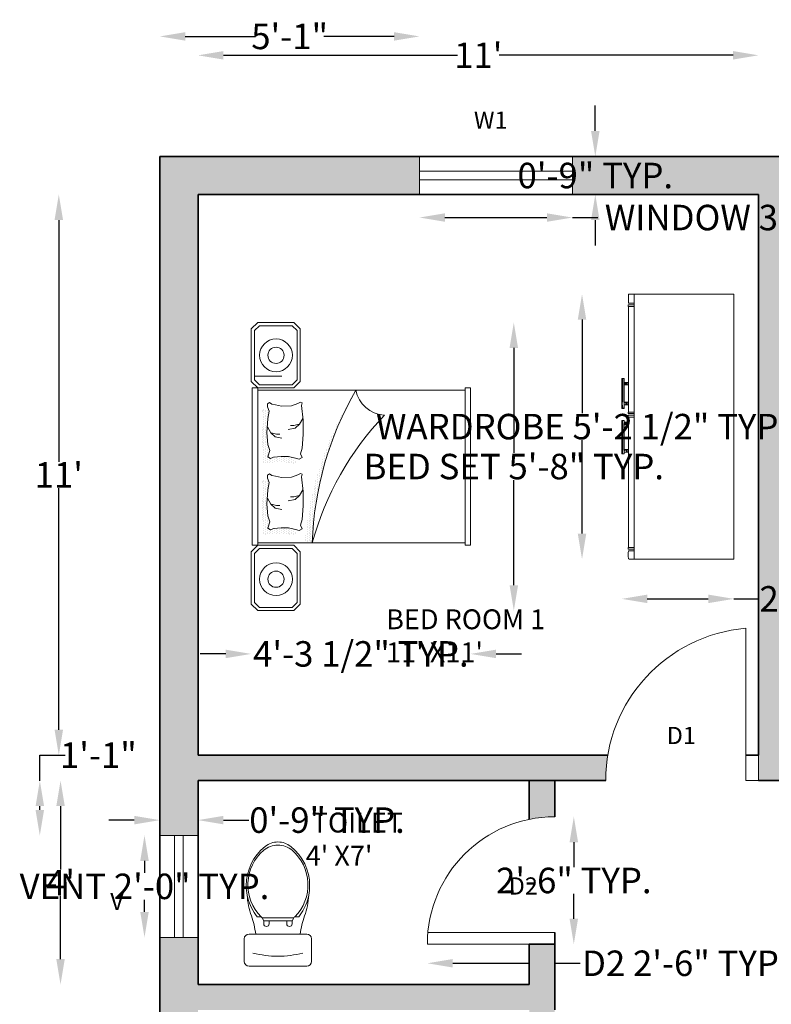
# Model space of a CAD drawing. Units: inches. Extents: x 2178 to 3409, y 1711 to 2279.
# Tile 3 of 8: x 2191 to 2368, y 2047 to 2279. Entities that reach past the tile are written whole.
import ezdxf

# ---------------------------------------------------------------- set-up
doc = ezdxf.new("R2010")
doc.units = ezdxf.units.IN
for name, color, linetype, lineweight in [('A-ANNO-DIMS', 2, 'Continuous', 18), ('A-ANNO-IDEN', 3, 'Continuous', 18), ('A-AREA-IDEN', 7, 'Continuous', 18), ('A-DOOR', 4, 'Continuous', 18), ('A-FURN', 8, 'Continuous', 18), ('A-GLAZ', 4, 'Continuous', 18), ('A-WALL', 7, 'Continuous', 35), ('A-WALL-PATT', 252, 'Continuous', 13), ('WC-Detail_dwgmodels.com', 240, 'Continuous', 13), ('WC-Outline_dwgmodels.com', 250, 'Continuous', 18)]:
    doc.layers.add(name, color=color, linetype=linetype, lineweight=lineweight)
doc.styles.get("Standard").update_dxf_attribs({"font": 'arial.ttf'})
doc.dimstyles.get("Standard").update_dxf_attribs({"dimtxt": 6, "dimasz": 6, "dimexe": 0.18, "dimexo": 0.0625, "dimgap": 0.09, "dimtad": 0, "dimtih": 1, "dimtoh": 1, "dimdec": 4, "dimzin": 0, "dimdsep": 46, "dimlunit": 4, "dimtxsty": 'Standard', "dimcen": 0.09, "dimse1": 1, "dimse2": 1, "dimadec": 0, "dimazin": 0, "dimtfac": 1, "dimtdec": 4, "dimtofl": 0, "dimtmove": 0, "dimatfit": 3, "dimfxl": 1, "dimtolj": 1, "dimtzin": 0, "dimarcsym": 0})
pattern_1 = [(90, (3285.2007, -5256.0159), (-0.408110856, 0.204055428), [0, -0.408110856])]
pattern_2 = [(2e-12, (221.4576, -2145.7372), (1.73228346, -0.78740157), [11.8110236, -1.574803, 3.937008, -0.7874016]), (2e-12, (222.5049, -2146.1309), (-0.7874016, -1.0472441), [2.3622047, -0.2598425, 4.7244094, -0.5905512]), (2e-12, (221.8513, -2146.4065), (4.09448819, -0.52755906), [6.2992126, -1.1023622, 3.1496063, -0.7874016])]

# ---------------------------------------------------------------- blocks, each defined once
blk = doc.blocks.new('*D11')
at = {"layer": 'A-ANNO-DIMS', "color": 0, "lineweight": -2, "transparency": 16777216}
for p, q in [((2200.28, 2232.04), (2200.28, 2175.14)), ((2200.28, 2112.04), (2200.28, 2168.94))]:
    blk.add_line(p, q, dxfattribs=at)
at = {"layer": 'A-ANNO-DIMS', "color": 0, "transparency": 16777216}
for points in [[(2199.28, 2232.04), (2201.28, 2232.04), (2200.28, 2238.04)], [(2199.28, 2112.04), (2201.28, 2112.04), (2200.28, 2106.04)]]:
    blk.add_solid(points, dxfattribs=at)
at = {"layer": 'Defpoints', "color": 0, "transparency": 16777216}
for p in [(2233.06, 2238.04), (2200.28, 2106.04), (2233.06, 2106.04)]:
    blk.add_point(p, dxfattribs=at)
at = {"layer": 'A-ANNO-DIMS', "color": 0, "transparency": 16777216, "insert": (2200.28, 2172.04), "char_height": 6, "attachment_point": 5}
blk.add_mtext("\\A1;11'", dxfattribs=at)
blk = doc.blocks.new('*D12')
at = {"layer": 'A-ANNO-DIMS', "color": 0, "lineweight": -2, "transparency": 16777216}
for p, q in [((2200.69, 2094.04), (2200.69, 2079.13)), ((2200.69, 2058.04), (2200.69, 2072.95))]:
    blk.add_line(p, q, dxfattribs=at)
at = {"layer": 'A-ANNO-DIMS', "color": 0, "transparency": 16777216}
for points in [[(2199.69, 2094.04), (2201.69, 2094.04), (2200.69, 2100.04)], [(2199.69, 2058.04), (2201.69, 2058.04), (2200.69, 2052.04)]]:
    blk.add_solid(points, dxfattribs=at)
at = {"layer": 'Defpoints', "color": 0, "transparency": 16777216}
for p in [(2275.48, 2100.04), (2200.69, 2052.04), (2275.48, 2052.04)]:
    blk.add_point(p, dxfattribs=at)
at = {"layer": 'A-ANNO-DIMS', "color": 0, "transparency": 16777216, "insert": (2200.69, 2076.04), "char_height": 6, "attachment_point": 5}
blk.add_mtext("\\A1;4'", dxfattribs=at)
blk = doc.blocks.new('*D19')
at = {"layer": 'A-ANNO-DIMS', "color": 0, "lineweight": -2, "transparency": 16777216}
for p, q in [((2239.06, 2270.84), (2294.17, 2270.84)), ((2359.06, 2270.84), (2303.96, 2270.84))]:
    blk.add_line(p, q, dxfattribs=at)
at = {"layer": 'A-ANNO-DIMS', "color": 0, "transparency": 16777216}
for points in [[(2239.06, 2271.84), (2239.06, 2269.84), (2233.06, 2270.84)], [(2359.06, 2271.84), (2359.06, 2269.84), (2365.06, 2270.84)]]:
    blk.add_solid(points, dxfattribs=at)
at = {"layer": 'Defpoints', "color": 0, "transparency": 16777216}
for p in [(2365.06, 2270.84), (2233.06, 2238.04), (2365.06, 2238.04)]:
    blk.add_point(p, dxfattribs=at)
at = {"layer": 'A-ANNO-DIMS', "color": 0, "transparency": 16777216, "insert": (2299.06, 2270.84), "char_height": 6, "attachment_point": 5}
blk.add_mtext("\\A1;11'", dxfattribs=at)
blk = doc.blocks.new('BED-WITH-NIGHTSTANDS')
h = blk.add_hatch()
h.set_pattern_fill('DOTS', color=256, scale=0.257078, angle=90, style=0)
h.set_pattern_definition(pattern_1)
h.paths.add_polyline_path([(12.63, 18.62), (14.4, 18.62, -0.124273), (24.68, 54.62, 0.122563)])
h = blk.add_hatch()
h.set_pattern_fill('DOTS', color=256, scale=0.257078, angle=90, style=0)
h.set_pattern_definition(pattern_1)
h.paths.add_polyline_path([(3.05, 33.63), (2.57, 33.32), (2.57, 32.61), (2.97, 31.58), (2.65, 29.84), (2.42, 26.52), (2.65, 23.75), (3.13, 22.32), (2.65, 20.82), (3.28, 20.43), (4, 20.74), (5.81, 20.9), (7.55, 20.9), (9.13, 20.51), (10, 20.27), (10.71, 20.66), (10.32, 21.53), (10.39, 21.79), (8.83, 22.19), (7.1, 22.19), (5.28, 22.03), (4.57, 21.71), (3.93, 22.11), (4.41, 23.61), (3.93, 25.03), (3.7, 27.8), (3.93, 31.12), (4.25, 32.86), (4.14, 33.14), (3.6, 33.24)])
h.paths.add_polyline_path([(3.05, 50.43), (2.57, 50.11), (2.57, 49.4), (2.97, 48.37), (2.65, 46.63), (2.42, 43.31), (2.65, 40.54), (3.13, 39.12), (2.65, 37.62), (3.28, 37.22), (4, 37.54), (5.81, 37.7), (7.55, 37.7), (9.13, 37.3), (10, 37.06), (10.71, 37.46), (10.32, 38.33), (10.39, 38.59), (8.83, 38.98), (7.1, 38.98), (5.28, 38.82), (4.57, 38.51), (3.93, 38.9), (4.41, 40.4), (3.93, 41.83), (3.7, 44.59), (3.93, 47.92), (4.25, 49.66), (4.14, 49.93), (3.6, 50.03)])
for p, q in [((0.8, 57.9), (7.23, 57.9)), ((0.26, 55.13), (0.26, 18.11)), ((0.26, 55.13), (1.54, 55.13)), ((1.54, 55.13), (1.54, 18.11)), ((1.54, 54.62), (50.39, 54.62)), ((50.39, 55.13), (50.39, 18.11)), ((50.39, 55.13), (51.67, 55.13)), ((51.67, 55.13), (51.67, 18.11)), ((50.39, 18.62), (1.54, 18.62)), ((1.54, 18.11), (0.26, 18.11)), ((51.67, 18.11), (50.39, 18.11))]:
    blk.add_line(p, q)
for points in [[(11.57, 56.67), (11.57, 69.01), (10.03, 70.55), (1.54, 70.55), (0, 69.01), (0, 56.67), (1.54, 55.13), (10.03, 55.13)], [(10.8, 57.06), (10.8, 68.63), (9.64, 69.78), (1.93, 69.78), (0.77, 68.63), (0.77, 57.06), (1.93, 55.9), (9.64, 55.9)], [(11.57, 4.23), (11.57, 16.57), (10.03, 18.11), (1.54, 18.11), (0, 16.57), (0, 4.23), (1.54, 2.69), (10.03, 2.69)], [(10.8, 4.61), (10.8, 16.18), (9.64, 17.34), (1.93, 17.34), (0.77, 16.18), (0.77, 4.61), (1.93, 3.46), (9.64, 3.46)]]:
    blk.add_lwpolyline(points, close=True)
for points in [[(4.41, 40.4), (3.93, 38.9), (4.57, 38.51), (5.28, 38.82), (7.1, 38.98), (8.83, 38.98), (10.41, 38.58), (11.28, 38.35), (11.99, 38.74), (11.6, 39.61), (11.99, 40.96), (12.23, 44.2), (12.23, 47.52), (11.84, 51), (11.99, 51.63), (11.6, 51.79), (10.97, 51.47), (9.54, 50.92), (7.17, 50.84), (5.75, 51.16), (4.88, 51.32), (4.33, 51.71), (3.86, 51.4), (3.86, 50.68), (4.25, 49.66), (3.93, 47.92), (3.7, 44.59), (3.93, 41.83), (4.41, 40.4)], [(12.15, 47.92), (11.36, 46.57), (10.33, 45.62), (8.75, 45.31)], [(11.28, 46.57), (10.02, 46.26), (9.23, 46.26)], [(3.86, 45.94), (4.65, 44.59), (5.67, 43.65), (7.25, 43.33)], [(4.72, 44.59), (5.99, 44.28), (6.78, 44.28)], [(4.41, 23.61), (3.93, 22.11), (4.57, 21.71), (5.28, 22.03), (7.1, 22.19), (8.83, 22.19), (10.41, 21.79), (11.28, 21.55), (11.99, 21.95), (11.6, 22.82), (11.99, 24.16), (12.23, 27.4), (12.23, 30.73), (11.84, 34.21), (11.99, 34.84), (11.6, 35), (10.97, 34.68), (9.54, 34.13), (7.17, 34.05), (5.75, 34.36), (4.88, 34.52), (4.33, 34.92), (3.86, 34.6), (3.86, 33.89), (4.25, 32.86), (3.93, 31.12), (3.7, 27.8), (3.93, 25.03), (4.41, 23.61)], [(12.15, 31.12), (11.36, 29.78), (10.33, 28.83), (8.75, 28.51)], [(3.86, 29.14), (4.65, 27.8), (5.67, 26.85), (7.25, 26.53)], [(11.28, 29.78), (10.02, 29.46), (9.23, 29.46)], [(4.72, 27.8), (5.99, 27.48), (6.78, 27.48)]]:
    blk.add_lwpolyline(points)
for centre, radius in [((5.86, 62.82), 3.86), ((5.86, 62.82), 1.91), ((5.86, 10.09), 3.86), ((5.86, 10.09), 1.91)]:
    blk.add_circle(centre, radius)
for centre, radius, start, end in [((90.82, 16.25), 76.46, 149.8866, 178.2226), ((31.77, 55.91), 7.21, 190.3543, 266.7862), ((82.59, 0), 70.69, 136.4367, 164.7234)]:
    blk.add_arc(centre, radius, start, end)
blk = doc.blocks.new('BEDROOM-WARDROBE')
h = blk.add_hatch()
h.set_pattern_fill('AR-RROOF', color=256, scale=0.787402, angle=360, style=0)
h.set_pattern_definition(pattern_2)
h.paths.add_polyline_path([(19.88, 0.59), (19.88, 0), (26.97, 0), (26.97, 0.59)])
h.paths.add_polyline_path([(26.07, 1.57), (25.48, 1.57), (25.48, 0.59), (26.07, 0.59)])
h.paths.add_polyline_path([(21.37, 1.57), (20.78, 1.57), (20.78, 0.59), (21.37, 0.59)])
h = blk.add_hatch()
h.set_pattern_fill('AR-RROOF', color=256, scale=0.787402, angle=360, style=0)
h.set_pattern_definition(pattern_2)
h.paths.add_polyline_path([(29.73, 0.59), (29.73, 0), (37.6, 0), (37.6, 0.59)])
h.paths.add_polyline_path([(37.21, 1.57), (36.61, 1.57), (36.61, 0.59), (37.21, 0.59)])
h.paths.add_polyline_path([(30.71, 0.59), (30.71, 1.57), (30.12, 1.57), (30.12, 0.59)])
for p, q in [((0, 26.38), (62.4, 26.38)), ((0, 26.38), (0, 1.57)), ((62.4, 26.38), (62.4, 1.74)), ((62.4, 2.95), (0, 2.95)), ((2.17, 1.57), (2.17, 2.95)), ((2.56, 1.54), (2.56, 2.95)), ((2.95, 1.57), (2.95, 2.95)), ((27.76, 2.95), (27.76, 1.57)), ((28.15, 2.95), (28.15, 1.54)), ((28.54, 2.95), (28.54, 1.54)), ((28.94, 2.95), (28.94, 1.57)), ((59.65, 2.95), (59.65, 1.57)), ((60.04, 1.54), (60.04, 2.95)), ((60.43, 2.95), (60.43, 1.57)), ((0, 1.57), (2.17, 1.57)), ((2.95, 1.54), (2.56, 1.54)), ((27.76, 1.57), (2.95, 1.57)), ((2.95, 1.57), (2.95, 1.54)), ((19.88, 0.59), (26.97, 0.59)), ((19.88, 0), (19.88, 0.59)), ((26.97, 0), (19.88, 0)), ((20.78, 0.59), (20.78, 1.57)), ((21.37, 0.59), (21.37, 1.57)), ((25.48, 0.59), (25.48, 1.57)), ((26.07, 0.59), (26.07, 1.57)), ((26.97, 0.59), (26.97, 0)), ((27.76, 1.54), (27.76, 1.57)), ((28.15, 1.54), (27.76, 1.54)), ((28.54, 1.54), (28.94, 1.54)), ((28.94, 1.57), (59.65, 1.57)), ((28.94, 1.54), (28.94, 1.57)), ((29.73, 0.59), (37.6, 0.59)), ((29.73, 0), (29.73, 0.59)), ((37.6, 0), (29.73, 0)), ((30.12, 0.59), (30.12, 1.57)), ((30.71, 0.59), (30.71, 1.57)), ((36.61, 0.59), (36.61, 1.57)), ((37.21, 0.59), (37.21, 1.57)), ((37.6, 0.59), (37.6, 0)), ((59.65, 1.57), (59.65, 1.54)), ((59.65, 1.54), (60.04, 1.54))]:
    blk.add_line(p, q)
for centre, radius, start, end in [((61.42, 6.59), 5.11, 258.8892, 279.227), ((62.2, 1.74), 0.197, 279.227, 0)]:
    blk.add_arc(centre, radius, start, end)
blk = doc.blocks.new('WC-SEAT-ASSEMBLY')
for p, q in [((3.53, 1.38), (3.89, 0.72)), ((5.18, 0.72), (3.89, 0.72)), ((3.89, 0.72), (3.89, 0)), ((7.25, 0.72), (5.18, 0.72)), ((5.18, 0), (5.18, 0.72)), ((7.25, 0.72), (9.32, 0.72)), ((9.32, 0.72), (10.61, 0.72)), ((9.32, 0), (9.32, 0.72)), ((10.97, 1.38), (10.61, 0.72)), ((10.61, 0.72), (10.61, 0))]:
    blk.add_line(p, q)
for points in [[(3.26, 1.65, -0.434217), (3.89, 17.29, -0.182634), (7.25, 18.51, -2.693815)], [(11.24, 1.65, 0.434217), (10.61, 17.29, 0.182634), (7.25, 18.51, 2.693815)], [(0.16, 6.03, -0.015301), (0, 6.73, -0.16845)], [(2.36, 1.65, -0.105447), (0.16, 6.03, -0.16845)], [(12.14, 1.65, 0.094048), (14.19, 5.52, 0.16845)], [(14.19, 5.52, 0.026594), (14.5, 6.73, 0.16845)], [(3.26, 1.65), (2.36, 1.65, -0.416606)], [(3.53, 1.38, -0.008985), (3.26, 1.65, -0.182634)], [(7.25, 1.38), (3.53, 1.38, -0.444938)], [(7.25, 1.38), (10.97, 1.38, 0.008985)], [(10.97, 1.38, 0.008985), (11.24, 1.65, 0.182634)], [(11.24, 1.65), (12.14, 1.65, 0.416606)]]:
    blk.add_lwpolyline(points, format="xyb")
for centre in [(4.54, 0), (9.96, 0)]:
    blk.add_arc(centre, 0.645, 180, 0)
blk = doc.blocks.new('WINDOW-36')
for p, q in [((36, 9), (0, 9)), ((0, 9), (0, 0)), ((36, 0), (36, 9)), ((0, 5.5), (36, 5.5)), ((0, 3.5), (36, 3.5)), ((0, 0), (36, 0))]:
    blk.add_line(p, q)
blk = doc.blocks.new('VENT-24')
for p, q in [((9, 24), (0, 24)), ((0, 24), (0, 0)), ((3.5, 0), (3.5, 24)), ((5.5, 0), (5.5, 24)), ((9, 0), (9, 24)), ((0, 0), (9, 0))]:
    blk.add_line(p, q)
blk = doc.blocks.new('DOOR-30')
for p, q in [((-30, 2.75), (0, 2.75)), ((0, 2.75), (0, 0)), ((-30, 0), (0, 0))]:
    blk.add_line(p, q)
blk.add_arc((0, 0), 30, 90, 180)
blk = doc.blocks.new('*D35')
at = {"layer": 'A-ANNO-DIMS', "color": 0, "lineweight": -2, "transparency": 16777216}
for p, q in [((2307.43, 2201.94), (2307.43, 2177.2)), ((2307.43, 2146.07), (2307.43, 2170.82))]:
    blk.add_line(p, q, dxfattribs=at)
at = {"layer": 'A-ANNO-DIMS', "color": 0, "transparency": 16777216}
for points in [[(2306.43, 2201.94), (2308.43, 2201.94), (2307.43, 2207.94)], [(2306.43, 2146.07), (2308.43, 2146.07), (2307.43, 2140.07)]]:
    blk.add_solid(points, dxfattribs=at)
at = {"layer": 'Defpoints', "color": 0, "transparency": 16777216}
for p in [(2297.25, 2207.94), (2307.43, 2207.94), (2297.25, 2140.07)]:
    blk.add_point(p, dxfattribs=at)
at = {"layer": 'A-ANNO-DIMS', "color": 0, "transparency": 16777216, "insert": (2307.43, 2174.01), "char_height": 6, "attachment_point": 5}
blk.add_mtext('\\A1;BED SET 5\'-8" TYP.', dxfattribs=at)
blk = doc.blocks.new('*D36')
at = {"layer": 'A-ANNO-DIMS', "color": 0, "lineweight": -2, "transparency": 16777216}
for p, q in [((2239.58, 2129.89), (2233.58, 2129.89)), ((2303.25, 2129.89), (2309.25, 2129.89))]:
    blk.add_line(p, q, dxfattribs=at)
at = {"layer": 'A-ANNO-DIMS', "color": 0, "transparency": 16777216}
for points in [[(2239.58, 2130.89), (2239.58, 2128.89), (2245.58, 2129.89)], [(2303.25, 2130.89), (2303.25, 2128.89), (2297.25, 2129.89)]]:
    blk.add_solid(points, dxfattribs=at)
at = {"layer": 'Defpoints', "color": 0, "transparency": 16777216}
for p in [(2245.58, 2140.07), (2297.25, 2140.07), (2297.25, 2129.89)]:
    blk.add_point(p, dxfattribs=at)
at = {"layer": 'A-ANNO-DIMS', "color": 0, "transparency": 16777216, "insert": (2271.41, 2129.89), "char_height": 6, "attachment_point": 5}
blk.add_mtext('\\A1;4\'-3 1/2" TYP.', dxfattribs=at)
blk = doc.blocks.new('*D37')
at = {"layer": 'A-ANNO-DIMS', "color": 0, "lineweight": -2, "transparency": 16777216}
for p, q in [((2323.49, 2208.61), (2323.49, 2186.6)), ((2323.49, 2158.21), (2323.49, 2180.22))]:
    blk.add_line(p, q, dxfattribs=at)
at = {"layer": 'A-ANNO-DIMS', "color": 0, "transparency": 16777216}
for points in [[(2322.49, 2208.61), (2324.49, 2208.61), (2323.49, 2214.61)], [(2322.49, 2158.21), (2324.49, 2158.21), (2323.49, 2152.21)]]:
    blk.add_solid(points, dxfattribs=at)
at = {"layer": 'Defpoints', "color": 0, "transparency": 16777216}
for p in [(2332.85, 2214.61), (2323.49, 2152.21), (2332.85, 2152.21)]:
    blk.add_point(p, dxfattribs=at)
at = {"layer": 'A-ANNO-DIMS', "color": 0, "transparency": 16777216, "insert": (2323.49, 2183.41), "char_height": 6, "attachment_point": 5}
blk.add_mtext('\\A1;WARDROBE 5\'-2 1/2" TYP.', dxfattribs=at)
blk = doc.blocks.new('*D38')
at = {"layer": 'A-ANNO-DIMS', "color": 0, "lineweight": -2, "transparency": 16777216}
for p, q in [((2338.85, 2142.85), (2353.23, 2142.85)), ((2359.23, 2142.85), (2365.23, 2142.85))]:
    blk.add_line(p, q, dxfattribs=at)
at = {"layer": 'A-ANNO-DIMS', "color": 0, "transparency": 16777216}
for points in [[(2338.85, 2143.85), (2338.85, 2141.85), (2332.85, 2142.85)], [(2353.23, 2143.85), (2353.23, 2141.85), (2359.23, 2142.85)]]:
    blk.add_solid(points, dxfattribs=at)
at = {"layer": 'Defpoints', "color": 0, "transparency": 16777216}
for p in [(2332.85, 2152.21), (2359.23, 2152.21), (2359.23, 2142.85)]:
    blk.add_point(p, dxfattribs=at)
at = {"layer": 'A-ANNO-DIMS', "color": 0, "transparency": 16777216, "insert": (2390.65, 2142.85), "char_height": 6, "attachment_point": 5}
blk.add_mtext('\\A1;2\'-2 1/2" TYP.', dxfattribs=at)
blk = doc.blocks.new('*D47')
at = {"layer": 'A-ANNO-DIMS', "color": 0, "lineweight": -2, "transparency": 16777216}
for p, q in [((2291.22, 2232.64), (2315.22, 2232.64)), ((2321.22, 2232.64), (2327.22, 2232.64))]:
    blk.add_line(p, q, dxfattribs=at)
at = {"layer": 'A-ANNO-DIMS', "color": 0, "transparency": 16777216}
for points in [[(2291.22, 2233.64), (2291.22, 2231.64), (2285.22, 2232.64)], [(2315.22, 2233.64), (2315.22, 2231.64), (2321.22, 2232.64)]]:
    blk.add_solid(points, dxfattribs=at)
at = {"layer": 'Defpoints', "color": 0, "transparency": 16777216}
for p in [(2285.22, 2238.04), (2321.22, 2238.04), (2321.22, 2232.64)]:
    blk.add_point(p, dxfattribs=at)
at = {"layer": 'A-ANNO-DIMS', "color": 0, "transparency": 16777216, "insert": (2365.28, 2232.64), "char_height": 6, "attachment_point": 5}
blk.add_mtext('\\A1;WINDOW 3\'-0" TYP.', dxfattribs=at)
blk = doc.blocks.new('*D48')
at = {"layer": 'A-ANNO-DIMS', "color": 0, "lineweight": -2, "transparency": 16777216}
for p, q in [((2326.62, 2253.04), (2326.62, 2259.04)), ((2326.62, 2232.04), (2326.62, 2226.04))]:
    blk.add_line(p, q, dxfattribs=at)
at = {"layer": 'A-ANNO-DIMS', "color": 0, "transparency": 16777216}
for points in [[(2325.62, 2253.04), (2327.62, 2253.04), (2326.62, 2247.04)], [(2325.62, 2232.04), (2327.62, 2232.04), (2326.62, 2238.04)]]:
    blk.add_solid(points, dxfattribs=at)
at = {"layer": 'Defpoints', "color": 0, "transparency": 16777216}
for p in [(2321.22, 2247.04), (2326.62, 2247.04), (2321.22, 2238.04)]:
    blk.add_point(p, dxfattribs=at)
at = {"layer": 'A-ANNO-DIMS', "color": 0, "transparency": 16777216, "insert": (2326.62, 2242.54), "char_height": 6, "attachment_point": 5}
blk.add_mtext('\\A1;0\'-9" TYP.', dxfattribs=at)
blk = doc.blocks.new('*D49')
at = {"layer": 'A-ANNO-DIMS', "color": 0, "lineweight": -2, "transparency": 16777216}
for p, q in [((2220.46, 2081.15), (2220.46, 2078.3)), ((2220.46, 2069.15), (2220.46, 2071.99))]:
    blk.add_line(p, q, dxfattribs=at)
at = {"layer": 'A-ANNO-DIMS', "color": 0, "transparency": 16777216}
for points in [[(2219.46, 2081.15), (2221.46, 2081.15), (2220.46, 2087.15)], [(2219.46, 2069.15), (2221.46, 2069.15), (2220.46, 2063.15)]]:
    blk.add_solid(points, dxfattribs=at)
at = {"layer": 'Defpoints', "color": 0, "transparency": 16777216}
for p in [(2220.46, 2087.15), (2224.06, 2087.15), (2224.06, 2063.15)]:
    blk.add_point(p, dxfattribs=at)
at = {"layer": 'A-ANNO-DIMS', "color": 0, "transparency": 16777216, "insert": (2220.46, 2075.15), "char_height": 6, "attachment_point": 5}
blk.add_mtext('\\A1;VENT 2\'-0" TYP.', dxfattribs=at)
blk = doc.blocks.new('*D50')
at = {"layer": 'A-ANNO-DIMS', "color": 0, "lineweight": -2, "transparency": 16777216}
for p, q in [((2218.06, 2090.75), (2212.06, 2090.75)), ((2239.06, 2090.75), (2245.06, 2090.75))]:
    blk.add_line(p, q, dxfattribs=at)
at = {"layer": 'A-ANNO-DIMS', "color": 0, "transparency": 16777216}
for points in [[(2218.06, 2091.75), (2218.06, 2089.75), (2224.06, 2090.75)], [(2239.06, 2091.75), (2239.06, 2089.75), (2233.06, 2090.75)]]:
    blk.add_solid(points, dxfattribs=at)
at = {"layer": 'Defpoints', "color": 0, "transparency": 16777216}
for p in [(2233.06, 2090.75), (2224.06, 2087.15), (2233.06, 2087.15)]:
    blk.add_point(p, dxfattribs=at)
at = {"layer": 'A-ANNO-DIMS', "color": 0, "transparency": 16777216, "insert": (2263.44, 2090.75), "char_height": 6, "attachment_point": 5}
blk.add_mtext('\\A1;0\'-9" TYP.', dxfattribs=at)
blk = doc.blocks.new('*D53')
at = {"layer": 'A-ANNO-DIMS', "color": 0, "lineweight": -2, "transparency": 16777216}
for p, q in [((2293.06, 2057.04), (2311.06, 2057.04)), ((2317.06, 2057.04), (2323.06, 2057.04))]:
    blk.add_line(p, q, dxfattribs=at)
at = {"layer": 'A-ANNO-DIMS', "color": 0, "transparency": 16777216}
for points in [[(2293.06, 2058.04), (2293.06, 2056.04), (2287.06, 2057.04)], [(2311.06, 2058.04), (2311.06, 2056.04), (2317.06, 2057.04)]]:
    blk.add_solid(points, dxfattribs=at)
at = {"layer": 'Defpoints', "color": 0, "transparency": 16777216}
for p in [(2287.06, 2061.54), (2317.06, 2061.54), (2317.06, 2057.04)]:
    blk.add_point(p, dxfattribs=at)
at = {"layer": 'A-ANNO-DIMS', "color": 0, "transparency": 16777216, "insert": (2347.81, 2057.04), "char_height": 6, "attachment_point": 5}
blk.add_mtext('\\A1;D2 2\'-6" TYP.', dxfattribs=at)
blk = doc.blocks.new('*D54')
at = {"layer": 'A-ANNO-DIMS', "color": 0, "lineweight": -2, "transparency": 16777216}
for p, q in [((2321.56, 2085.54), (2321.56, 2079.7)), ((2321.56, 2067.54), (2321.56, 2073.39))]:
    blk.add_line(p, q, dxfattribs=at)
at = {"layer": 'A-ANNO-DIMS', "color": 0, "transparency": 16777216}
for points in [[(2320.56, 2085.54), (2322.56, 2085.54), (2321.56, 2091.54)], [(2320.56, 2067.54), (2322.56, 2067.54), (2321.56, 2061.54)]]:
    blk.add_solid(points, dxfattribs=at)
at = {"layer": 'Defpoints', "color": 0, "transparency": 16777216}
for p in [(2317.06, 2091.54), (2321.56, 2091.54), (2317.06, 2061.54)]:
    blk.add_point(p, dxfattribs=at)
at = {"layer": 'A-ANNO-DIMS', "color": 0, "transparency": 16777216, "insert": (2321.56, 2076.54), "char_height": 6, "attachment_point": 5}
blk.add_mtext('\\A1;2\'-6" TYP.', dxfattribs=at)
blk = doc.blocks.new('*D62')
at = {"layer": 'A-ANNO-DIMS', "color": 0, "lineweight": -2, "transparency": 16777216}
for p, q in [((2195.81, 2100.04), (2195.81, 2106.04)), ((2195.81, 2106.04), (2201.81, 2106.04)), ((2195.81, 2093.15), (2195.81, 2094.04))]:
    blk.add_line(p, q, dxfattribs=at)
at = {"layer": 'A-ANNO-DIMS', "color": 0, "transparency": 16777216}
for points in [[(2194.81, 2094.04), (2196.81, 2094.04), (2195.81, 2100.04)], [(2194.81, 2093.15), (2196.81, 2093.15), (2195.81, 2087.15)]]:
    blk.add_solid(points, dxfattribs=at)
at = {"layer": 'Defpoints', "color": 0, "transparency": 16777216}
for p in [(2195.81, 2100.04), (2233.06, 2100.04), (2233.06, 2087.15)]:
    blk.add_point(p, dxfattribs=at)
at = {"layer": 'A-ANNO-DIMS', "color": 0, "transparency": 16777216, "insert": (2209.6, 2106.04), "char_height": 6, "attachment_point": 5}
blk.add_mtext('\\A1;1\'-1"', dxfattribs=at)
blk = doc.blocks.new('*D64')
at = {"layer": 'A-ANNO-DIMS', "color": 0, "lineweight": -2, "transparency": 16777216}
for p, q in [((2230.06, 2275.29), (2246.58, 2275.29)), ((2279.22, 2275.29), (2262.71, 2275.29))]:
    blk.add_line(p, q, dxfattribs=at)
at = {"layer": 'A-ANNO-DIMS', "color": 0, "transparency": 16777216}
for points in [[(2230.06, 2276.29), (2230.06, 2274.29), (2224.06, 2275.29)], [(2279.22, 2276.29), (2279.22, 2274.29), (2285.22, 2275.29)]]:
    blk.add_solid(points, dxfattribs=at)
at = {"layer": 'Defpoints', "color": 0, "transparency": 16777216}
for p in [(2285.22, 2275.29), (2224.06, 2247.04), (2285.22, 2247.04)]:
    blk.add_point(p, dxfattribs=at)
at = {"layer": 'A-ANNO-DIMS', "color": 0, "transparency": 16777216, "insert": (2254.64, 2275.29), "char_height": 6, "attachment_point": 5}
blk.add_mtext('\\A1;5\'-1"', dxfattribs=at)

msp = doc.modelspace()

# ---------------------------------------------------------------- hatches: boundary and pattern name
at = {"layer": 'A-WALL-PATT'}
h = msp.add_hatch(color=256, dxfattribs=at)
h.dxf.hatch_style = 1
h.paths.add_polyline_path([(2233.06485, 1992.04256), (2317.06485, 1992.04256), (2317.06485, 1998.04256), (2317.06485, 2006.75072), (2311.06485, 2006.75072), (2311.06485, 1998.04256), (2233.06485, 1998.04256), (2233.06485, 2009.64251), (2224.06485, 2009.64251), (2224.06485, 1863.04256), (2233.06485, 1863.04256), (2278.65041, 1863.04256), (2278.65041, 1872.04256), (2233.06485, 1872.04256)])
h.paths.add_polyline_path([(2359.06485, 1992.04256), (2359.06485, 1998.04256), (2353.06485, 1998.04256), (2353.06485, 1962.04256), (2353.06485, 1872.04256), (2314.65041, 1872.04256), (2314.65041, 1863.04256), (2359.06485, 1863.04256), (2359.06485, 1872.04256)])
h.paths.add_polyline_path([(2401.06485, 1890.04256), (2371.06485, 1890.04256), (2359.06485, 1890.04256), (2359.06485, 1884.04256), (2371.06485, 1884.04256), (2377.06485, 1884.04256), (2401.06485, 1884.04256)])
h.paths.add_polyline_path([(2353.06485, 1802.77269), (2359.06485, 1802.77269), (2359.06485, 1808.77269), (2356.83755, 1808.77269), (2353.06485, 1808.77269), (2347.91295, 1808.77269), (2347.91295, 1802.77269), (2347.91295, 1749.04256), (2342.02347, 1749.04256), (2342.02347, 1743.04256), (2353.06485, 1743.04256)])
h.paths.add_polyline_path([(2476.06485, 2247.04256), (2442.91353, 2247.04256), (2442.91353, 2238.04256), (2467.06485, 2238.04256), (2467.06485, 2041.93675), (2476.06485, 2041.93675)])
h.paths.add_polyline_path([(2467.06485, 2106.04256), (2406.56133, 2106.04256, -0.04188649), (2407.06485, 2100.04256), (2467.06485, 2100.04256)])
h.paths.add_polyline_path([(2406.91353, 2247.04256), (2321.22384, 2247.04256), (2321.22384, 2238.04256), (2365.06485, 2238.04256), (2365.06485, 2106.04256), (2365.06485, 2100.04256), (2371.06485, 2100.04256), (2371.06485, 2136.04256), (2371.06485, 2238.04256), (2406.91353, 2238.04256)])
h.paths.add_polyline_path([(2285.22384, 2247.04256), (2224.06485, 2247.04256), (2224.06485, 2087.1459), (2233.06485, 2087.1459), (2233.06485, 2100.04256), (2329.06485, 2100.04256, -0.04188649), (2329.56837, 2106.04256), (2233.06485, 2106.04256), (2233.06485, 2238.04256), (2285.22384, 2238.04256)])
h.paths.add_polyline_path([(2317.06485, 2052.04256), (2317.06485, 2061.5418), (2311.06485, 2061.5418), (2311.06485, 2052.04256), (2233.06485, 2052.04256), (2233.06485, 2063.1459), (2224.06485, 2063.1459), (2224.06485, 2033.64251), (2233.06485, 2033.64251), (2233.06485, 2046.04256), (2311.06485, 2046.04256), (2311.06485, 2036.1446, -0.050382044), (2317.06485, 2036.75072), (2317.06485, 2046.04256)])
h = msp.add_hatch(color=256, dxfattribs=at)
h.dxf.hatch_style = 1
h.paths.add_polyline_path([(2317.06485, 2100.04256), (2311.06485, 2100.04256), (2311.06485, 2090.93568, -0.050382044), (2317.06485, 2091.5418)])

# ---------------------------------------------------------------- linework, layer by layer
at = {"layer": 'A-DOOR'}
for p, q in [((2362.06485, 2106.04256), (2362.06485, 2135.91735)), ((2365.06485, 2100.04256), (2365.06485, 2136.04256)), ((2362.06485, 2106.04256), (2362.06485, 2100.04256)), ((2362.06485, 2100.04256), (2365.06485, 2100.04256)), ((2362.06485, 2100.04256), (2365.06485, 2100.04256))]:
    msp.add_line(p, q, dxfattribs=at)
msp.add_arc((2365.06485, 2100.04256), 36, 94.7801918, 180, dxfattribs=at)
at = {"layer": 'A-WALL'}
for p, q in [((2224.06485, 2247.04256), (2224.06485, 1863.04256)), ((2224.06485, 2247.04256), (2476.06485, 2247.04256)), ((2233.06485, 2238.04256), (2233.06485, 2106.04256)), ((2233.06485, 2238.04256), (2365.06485, 2238.04256)), ((2365.06485, 2238.04256), (2365.06485, 2106.04256)), ((2233.06485, 2106.04256), (2329.56837, 2106.04256)), ((2362.06485, 2106.04256), (2365.06485, 2106.04256)), ((2233.06485, 2100.04256), (2329.06485, 2100.04256)), ((2233.06485, 2100.04256), (2233.06485, 2052.04256)), ((2311.06485, 2100.04256), (2311.06485, 2090.93568)), ((2317.06485, 2100.04256), (2317.06485, 2091.5418)), ((2365.06485, 2100.04256), (2371.06485, 2100.04256)), ((2317.06485, 2064.2918), (2317.06485, 2052.04256)), ((2311.06485, 2061.5418), (2317.06485, 2061.5418)), ((2311.06485, 2061.5418), (2311.06485, 2052.04256)), ((2233.06485, 2052.04256), (2311.06485, 2052.04256)), ((2317.06485, 2052.04256), (2317.06485, 2046.04256))]:
    msp.add_line(p, q, dxfattribs=at)
at = {"layer": 'WC-Detail_dwgmodels.com'}
for centre, start, end in [((2251.89589, 2081.95688), 255.3287681, 269.9720383), ((2251.87319, 2081.95688), 270.0279617, 284.6712319)]:
    msp.add_arc(centre, 23.26046, start, end, dxfattribs=at)
at = {"layer": 'WC-Outline_dwgmodels.com'}
for points in [[(2244.41381, 2075.31603, -0.230343354), (2248.88531, 2084.56628, -0.168450027), (2251.88454, 2085.6069, -2.883081922)], [(2259.35528, 2075.31603, 0.230343354), (2254.88377, 2084.56628, 0.168450027), (2251.88454, 2085.6069, 2.883081922)], [(2244.63509, 2073.07646, -0.048022765), (2244.41381, 2075.31603, -0.168450027)], [(2259.13399, 2073.07646, 0.048022765), (2259.35528, 2075.31603, 0.168450027)], [(2245.09411, 2063.92807, 0.414213562), (2243.95593, 2062.78988), (2243.95593, 2057.48448, 0.414213562), (2245.09411, 2056.3463), (2251.88454, 2056.3463), (2258.67497, 2056.3463, 0.414213562), (2259.81316, 2057.48448), (2259.81316, 2062.78988, 0.414213562), (2258.67497, 2063.92807), (2257.11956, 2063.92807, -0.052345057), (2258.14382, 2068.17386, 0.071131414), (2259.13399, 2073.07646, 0.160777477)], [(2244.63509, 2073.07646, 0.071131414), (2245.62527, 2068.17386, -0.052345057), (2246.64953, 2063.92807), (2245.09411, 2063.92807, 0.414213562)], [(2246.64953, 2063.92807), (2251.88454, 2063.92807, -0.414213562)], [(2257.11956, 2063.92807), (2251.88454, 2063.92807, 0.414213562)]]:
    msp.add_lwpolyline(points, format="xyb", dxfattribs=at)

# ---------------------------------------------------------------- block references
at = {"layer": 'A-DOOR'}
msp.add_blockref('DOOR-30', (2317.06485, 2061.5418), dxfattribs=at)
at = {"layer": 'A-FURN', "rotation": 269.9999999999981}
msp.add_blockref('BEDROOM-WARDROBE', (2332.85429, 2214.61099), dxfattribs=at)
at = {"layer": 'A-FURN'}
msp.add_blockref('BED-WITH-NIGHTSTANDS', (2245.57589, 2137.38783), dxfattribs=at)
at = {"layer": 'A-GLAZ'}
for name, p in [('WINDOW-36', (2285.22384, 2238.04256)), ('VENT-24', (2224.06485, 2063.1459))]:
    msp.add_blockref(name, p, dxfattribs=at)
at = {"layer": 'WC-Detail_dwgmodels.com'}
msp.add_blockref('WC-SEAT-ASSEMBLY', (2244.63509, 2066.34944), dxfattribs=at)

# ---------------------------------------------------------------- texts
at = {"layer": 'A-ANNO-IDEN', "attachment_point": 1}
for s, insert, char_height in [('W1', (2298.02868, 2257.59918), 4.051205), ('D1', (2343.44445, 2112.7087), 4.051205), ('D2', (2306.21982, 2077.26875), 4.051205), ('V', (2212.39506, 2073.6249), 4.05121)]:
    msp.add_mtext_dynamic_manual_height_columns(s, width=167.0263497, gutter_width=20.25603, heights=[0], dxfattribs=dict(at, insert=insert, char_height=char_height))
at = {"layer": 'A-AREA-IDEN', "char_height": 4.679699, "attachment_point": 1}
for s, insert in [("BED ROOM 1\\P11' X11'", (2277.35594, 2140.38079)), (" TOILET\\P4' X7'", (2258.41544, 2092.51422))]:
    msp.add_mtext_dynamic_manual_height_columns(s, width=123.0595467, gutter_width=23.3985, heights=[41.64659], dxfattribs=dict(at, insert=insert))

# ---------------------------------------------------------------- dimensions: what is measured, and where the dimension line sits
at = {"layer": 'A-ANNO-DIMS'}
for base, p1, p2, override, picture, middle in [((2285.22384, 2275.29256), (2224.06485, 2247.04256), (2285.22384, 2247.04256), {"dimdec": 1, "dimlfac": 1, "dimrnd": 0, "dimzin": 1, "dimdsep": 46, "dimlunit": 4, "dimfrac": 2}, '*D64', (2254.64434, 2275.29256)), ((2365.06485, 2270.8418), (2233.06485, 2238.04256), (2365.06485, 2238.04256), {"dimclrd": 0, "dimclre": 0, "dimclrt": 0}, '*D19', (2299.06485, 2270.8418))]:
    dim = msp.add_linear_dim(base=base, p1=p1, p2=p2, dimstyle='Standard', override=override, dxfattribs=at)
    dim.commit()
    dim.dimension.update_dxf_attribs({"geometry": picture, "text_midpoint": middle})
for base, p1, p2, angle, text, picture, middle in [((2326.62384, 2247.04256), (2321.22384, 2238.04256), (2321.22384, 2247.04256), 90, '<> TYP.', '*D48', (2326.62384, 2242.54256)), ((2323.49406, 2152.20941), (2332.85429, 2214.61099), (2332.85429, 2152.20941), 270, 'WARDROBE <> TYP.', '*D37', (2323.49406, 2183.4102)), ((2307.42878, 2207.9425), (2297.24851, 2140.07399), (2297.24851, 2207.9425), 90, 'BED SET <> TYP.', '*D35', (2307.42878, 2174.00825)), ((2321.56485, 2091.5418), (2317.06485, 2061.5418), (2317.06485, 2091.5418), 90, '<> TYP.', '*D54', (2321.56485, 2076.5418)), ((2220.46485, 2087.1459), (2224.06485, 2063.1459), (2224.06485, 2087.1459), 90, 'VENT <> TYP.', '*D49', (2220.46485, 2075.1459))]:
    dim = msp.add_linear_dim(base=base, p1=p1, p2=p2, angle=angle, text=text, dimstyle='Standard', override={"dimdec": 1, "dimlfac": 1, "dimrnd": 0, "dimzin": 1, "dimdsep": 46, "dimlunit": 4, "dimfrac": 2}, dxfattribs=at)
    dim.commit()
    dim.dimension.update_dxf_attribs({"geometry": picture, "text_midpoint": middle})
for base, p1, p2, text, picture, middle in [((2321.22384, 2232.64256), (2285.22384, 2238.04256), (2321.22384, 2238.04256), 'WINDOW <> TYP.', '*D47', (2365.27632, 2232.64256)), ((2359.23207, 2142.84918), (2332.85429, 2152.20941), (2359.23207, 2152.20941), '<> TYP.', '*D38', (2390.65017, 2142.84918)), ((2297.24851, 2129.89371), (2245.57589, 2140.07399), (2297.24851, 2140.07399), '<> TYP.', '*D36', (2271.4122, 2129.89371)), ((2233.06485, 2090.7459), (2224.06485, 2087.1459), (2233.06485, 2087.1459), '<> TYP.', '*D50', (2263.44134, 2090.7459)), ((2317.06485, 2057.0418), (2287.06485, 2061.5418), (2317.06485, 2061.5418), 'D2 <> TYP.', '*D53', (2347.81378, 2057.0418))]:
    dim = msp.add_linear_dim(base=base, p1=p1, p2=p2, text=text, dimstyle='Standard', override={"dimdec": 1, "dimlfac": 1, "dimrnd": 0, "dimzin": 1, "dimdsep": 46, "dimlunit": 4, "dimfrac": 2}, dxfattribs=at)
    dim.commit()
    dim.dimension.update_dxf_attribs({"geometry": picture, "text_midpoint": middle})
for base, p1, p2, override, picture, middle in [((2200.27514, 2106.04256), (2233.06485, 2238.04256), (2233.06485, 2106.04256), {"dimclrd": 0, "dimclre": 0, "dimclrt": 0}, '*D11', (2200.27514, 2172.04256)), ((2195.81485, 2100.04256), (2233.06485, 2087.1459), (2233.06485, 2100.04256), {"dimdec": 1, "dimlfac": 1, "dimrnd": 0, "dimzin": 1, "dimdsep": 46, "dimlunit": 4, "dimfrac": 2}, '*D62', (2209.59721, 2106.04256)), ((2200.68963, 2052.04256), (2275.48496, 2100.04256), (2275.48496, 2052.04256), {"dimclrd": 0, "dimclre": 0, "dimclrt": 0}, '*D12', (2200.68963, 2076.04256))]:
    dim = msp.add_linear_dim(base=base, p1=p1, p2=p2, angle=90, dimstyle='Standard', override=override, dxfattribs=at)
    dim.commit()
    dim.dimension.update_dxf_attribs({"geometry": picture, "text_midpoint": middle})

doc.saveas('drawing.dxf')
